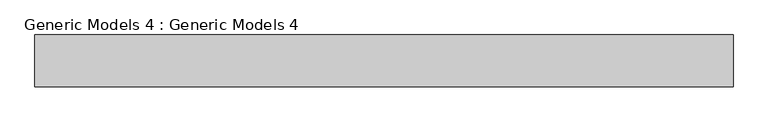
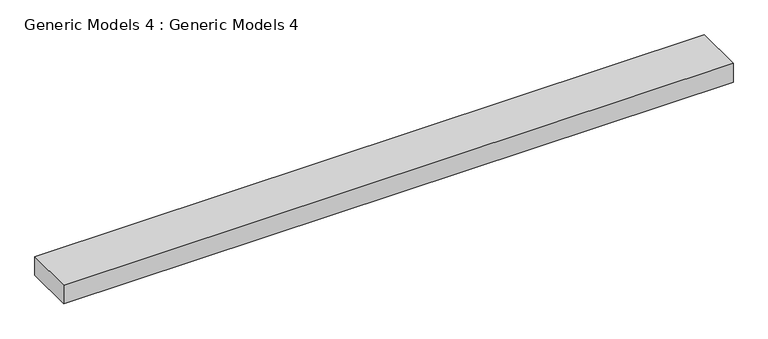
"""IFC4 building model written with IfcOpenShell, lengths in millimetres: proxy geometry, Generic Models 4 : Generic Models 4."""

from ifc_helpers import new_model, si_unit, frame, origin, place, context, project, spatial, polyline, outline, extrude, source, transform, mapped, element, save


def generic_models_4_generic_models_4_efb5897f(model_context):
    return source(origin(), model_context, "Body", "SweptSolid", [
        extrude(outline(polyline([(-7701.088074, -21683.9985361), (-7701.088074, -20921.9985361), (2581.2949202, -20921.9985361), (2581.2949202, -21683.9985361), (-7701.088074, -21683.9985361)])), frame((0.0, 0.0, 26517.6), z_axis=(0.0, 0.0, 1.0), x_axis=(1.0, 0.0, 0.0)), (0.0, 0.0, 1.0), 304.8),
    ])


if __name__ == "__main__":
    model = new_model("IFC4")
    model_context = context("Model", 3, world=origin())
    ifc_project = project(units=[si_unit("LENGTHUNIT", "METRE", prefix="MILLI")], contexts=[model_context])
    site = spatial("IfcSite", under=ifc_project)
    building = spatial("IfcBuilding", under=site)
    placement = place(None, origin())
    generic_models_4_generic_models_4_shape = generic_models_4_generic_models_4_efb5897f(model_context)
    element("IfcBuildingElementProxy", 1, Name="Generic Models 4 : Generic Models 4", ObjectType="Generic Models 4 : Generic Models 4", at=placement, inside=building, context=model_context, shape_type="MappedRepresentation", body=[
        mapped(generic_models_4_generic_models_4_shape, transform((0.0, 0.0, 0.0), x_axis=(1.0, 0.0, 0.0), y_axis=(0.0, 1.0, 0.0), z_axis=(0.0, 0.0, 1.0))),
    ])
    save(model, "model.ifc")
